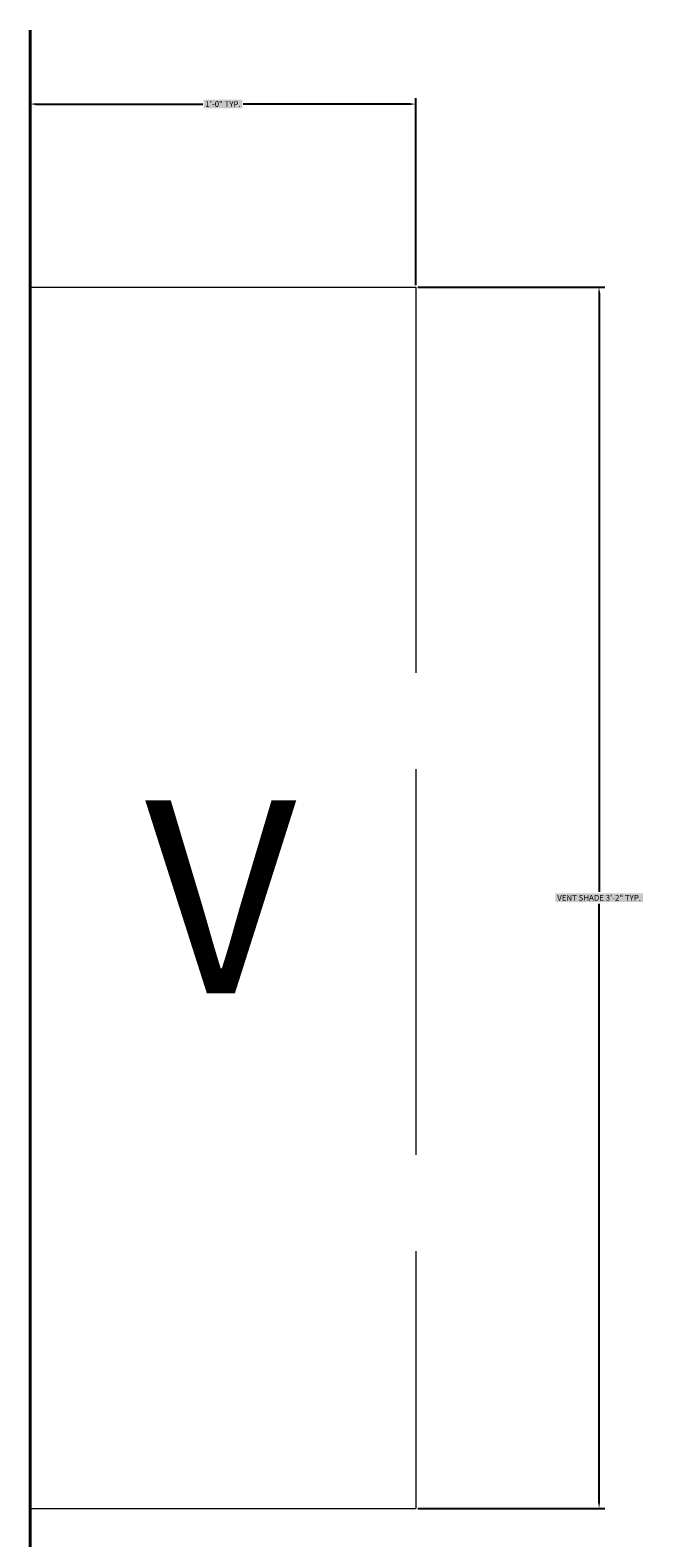
# Model space of a CAD drawing. Units: inches. Extents: x -301 to 715, y -607 to 364.
# Tile 95 of 141: x 133 to 152, y -124 to -77. Entities that reach past the tile are written whole.
import ezdxf

# ---------------------------------------------------------------- set-up
doc = ezdxf.new("R2010")
doc.units = ezdxf.units.IN
doc.header["$MEASUREMENT"] = 0
doc.linetypes.add('ACAD_ISO02W100', pattern=[15, 12, -3])
for name, color, linetype, lineweight in [('A-ANNO-DIMS', 2, 'Continuous', 18), ('A-ANNO-TEXT', 4, 'Continuous', 18), ('A-GLAZ-OVHD', 2, 'ACAD_ISO02W100', 18), ('A-WALL', 3, 'Continuous', 40)]:
    doc.layers.add(name, color=color, linetype=linetype, lineweight=lineweight)
doc.styles.get("Standard").update_dxf_attribs({"font": 'arial.ttf'})
doc.dimstyles.get("Standard").update_dxf_attribs({"dimtxt": 0.18, "dimasz": 0.18, "dimexe": 0.18, "dimexo": 0.0625, "dimgap": 0.09, "dimtad": 0, "dimtih": 1, "dimtoh": 1, "dimdec": 1, "dimzin": 0, "dimdsep": 46, "dimlunit": 4, "dimtxsty": 'Standard', "dimcen": 0.09, "dimclrd": 3, "dimclre": 4, "dimclrt": 6, "dimadec": 0, "dimazin": 0, "dimtfac": 1, "dimtdec": 1, "dimtofl": 0, "dimtmove": 0, "dimatfit": 3, "dimfxl": 1, "dimtfill": 2, "dimtfillclr": 51, "dimtolj": 1, "dimtzin": 0, "dimarcsym": 0})

# ---------------------------------------------------------------- blocks, each defined once
blk = doc.blocks.new('VENT-SHADE-38')
for p, q in [((0, 0), (0, 12)), ((0, 12), (38, 12)), ((38, 0), (38, 12)), ((5, 0), (0, 0)), ((33, 0), (38, 0))]:
    blk.add_line(p, q)
blk = doc.blocks.new('*D102')
at = {"layer": 'A-ANNO-DIMS', "color": 4, "lineweight": -2, "transparency": 16777216}
for p, q in [((144.959, -84.818), (150.777, -84.818)), ((144.959, -122.818), (150.777, -122.818))]:
    blk.add_line(p, q, dxfattribs=at)
at = {"layer": 'A-ANNO-DIMS', "color": 3, "lineweight": -2, "transparency": 16777216}
for p, q in [((150.597, -84.998), (150.597, -103.635)), ((150.597, -122.638), (150.597, -104.001))]:
    blk.add_line(p, q, dxfattribs=at)
at = {"layer": 'A-ANNO-DIMS', "color": 3, "transparency": 16777216}
for points in [[(150.567, -84.998), (150.627, -84.998), (150.597, -84.818)], [(150.567, -122.638), (150.627, -122.638), (150.597, -122.818)]]:
    blk.add_solid(points, dxfattribs=at)
at = {"layer": 'Defpoints', "color": 0, "transparency": 16777216}
for p in [(144.897, -84.818), (144.897, -122.818), (150.597, -122.818)]:
    blk.add_point(p, dxfattribs=at)
at = {"layer": 'A-ANNO-DIMS', "color": 6, "transparency": 16777216, "insert": (150.597, -103.818), "char_height": 0.18, "attachment_point": 5, "bg_fill": 1, "box_fill_scale": 1.25, "bg_fill_color": 51, "bg_fill_transparency": 0}
blk.add_mtext('\\A1;VENT SHADE 3\'-2" TYP.', dxfattribs=at)
blk = doc.blocks.new('*D103')
at = {"layer": 'A-ANNO-DIMS', "color": 4, "lineweight": -2, "transparency": 16777216}
for p, q in [((132.897, -84.755), (132.897, -78.938)), ((144.897, -84.755), (144.897, -78.938))]:
    blk.add_line(p, q, dxfattribs=at)
at = {"layer": 'A-ANNO-DIMS', "color": 3, "lineweight": -2, "transparency": 16777216}
for p, q in [((133.077, -79.118), (138.267, -79.118)), ((144.717, -79.118), (139.527, -79.118))]:
    blk.add_line(p, q, dxfattribs=at)
at = {"layer": 'A-ANNO-DIMS', "color": 3, "transparency": 16777216}
for points in [[(133.077, -79.088), (133.077, -79.148), (132.897, -79.118)], [(144.717, -79.088), (144.717, -79.148), (144.897, -79.118)]]:
    blk.add_solid(points, dxfattribs=at)
at = {"layer": 'Defpoints', "color": 0, "transparency": 16777216}
for p in [(144.897, -79.118), (132.897, -84.818), (144.897, -84.818)]:
    blk.add_point(p, dxfattribs=at)
at = {"layer": 'A-ANNO-DIMS', "color": 6, "transparency": 16777216, "insert": (138.897, -79.118), "char_height": 0.18, "attachment_point": 5, "bg_fill": 1, "box_fill_scale": 1.25, "bg_fill_color": 51, "bg_fill_transparency": 0}
blk.add_mtext('\\A1;1\'-0" TYP.', dxfattribs=at)

msp = doc.modelspace()

# ---------------------------------------------------------------- linework, layer by layer
at = {"layer": 'A-WALL'}
msp.add_line((132.897, -124.818), (132.897, -76.818), dxfattribs=at)

# ---------------------------------------------------------------- block references
at = {"layer": 'A-GLAZ-OVHD', "rotation": 269.9999999999998}
msp.add_blockref('VENT-SHADE-38', (132.896, -84.818), dxfattribs=at)

# ---------------------------------------------------------------- texts
at = {"layer": 'A-ANNO-TEXT'}
msp.add_text('V', height=6, dxfattribs=at).set_placement((136.469, -106.785))

# ---------------------------------------------------------------- dimensions: what is measured, and where the dimension line sits
at = {"layer": 'A-ANNO-DIMS'}
dim = msp.add_linear_dim(base=(144.897, -79.118), p1=(132.897, -84.818), p2=(144.897, -84.818), text='<> TYP.', dimstyle='Standard', override={"dimdec": 1, "dimlfac": 1, "dimrnd": 0, "dimzin": 1, "dimdsep": 46, "dimlunit": 4, "dimfrac": 2}, dxfattribs=at)
dim.commit()
dim.dimension.update_dxf_attribs({"geometry": '*D103', "text_midpoint": (138.897, -79.118)})
dim = msp.add_linear_dim(base=(150.597, -122.818), p1=(144.897, -84.818), p2=(144.897, -122.818), angle=270, text='VENT SHADE <> TYP.', dimstyle='Standard', override={"dimdec": 1, "dimlfac": 1, "dimrnd": 0, "dimzin": 1, "dimdsep": 46, "dimlunit": 4, "dimfrac": 2}, dxfattribs=at)
dim.commit()
dim.dimension.update_dxf_attribs({"geometry": '*D102', "text_midpoint": (150.597, -103.818)})

doc.saveas('drawing.dxf')
